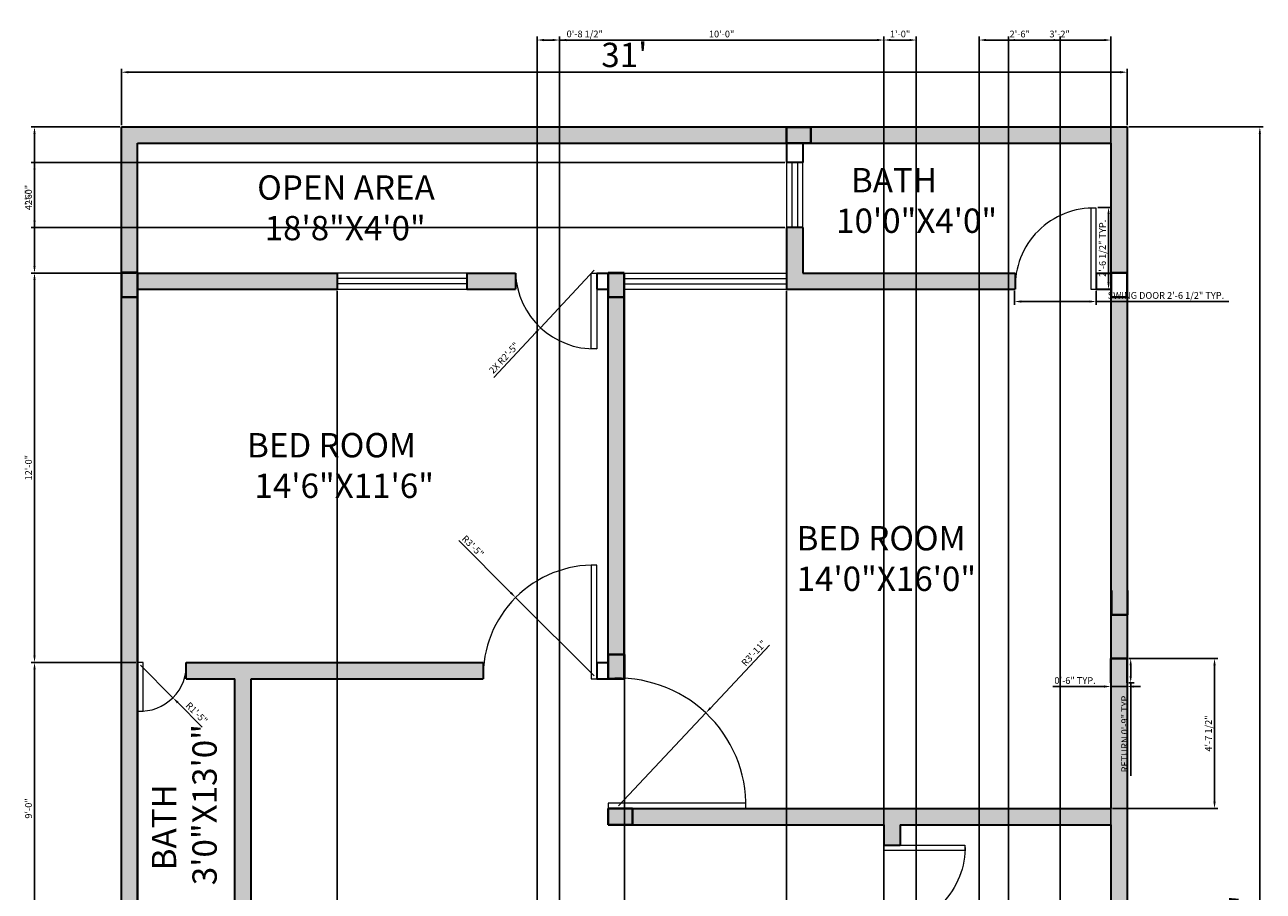
# Model space of a CAD drawing. Units: inches. Extents: x 5276 to 5736, y 3292 to 3966.
# Tile 3 of 3: x 5278 to 5736, y 3646 to 3966. Entities that reach past the tile are written whole.
import ezdxf

# ---------------------------------------------------------------- set-up
doc = ezdxf.new("R2010")
doc.units = ezdxf.units.IN
for name, color, linetype, lineweight in [('A-ANNO-DIMS', 2, 'Continuous', 18), ('A-AREA-IDEN', 7, 'Continuous', 18), ('A-COLS', 7, 'Continuous', 40), ('A-DOOR', 3, 'Continuous', 18), ('A-GLAZ', 4, 'Continuous', 18), ('A-WALL', 7, 'Continuous', 35)]:
    doc.layers.add(name, color=color, linetype=linetype, lineweight=lineweight)
doc.layers.add('A-COLS-PATT', color=244, linetype='Continuous', lineweight=13, true_color=0x991b1e)
doc.layers.add('A-WALL-PATT', color=141, linetype='Continuous', lineweight=13, true_color=0xadddf7)
doc.styles.get("Standard").update_dxf_attribs({"font": 'arial.ttf'})
doc.dimstyles.new('ISO-25', dxfattribs={"dimtxt": 2.5, "dimasz": 2.5, "dimexe": 1.25, "dimexo": 0.625, "dimtad": 1, "dimlunit": 3, "dimtxsty": 'Standard', "dimcen": 2.5, "dimadec": 0, "dimazin": 0, "dimtfac": 1, "dimtmove": 0, "dimatfit": 3, "dimfxl": 1, "dimarcsym": 0})

# ---------------------------------------------------------------- blocks, each defined once
blk = doc.blocks.new('*D16')
at = {"layer": 'A-ANNO-DIMS', "color": 0, "lineweight": -2, "transparency": 16777216}
for p, q in [((5314.13, 3928.87), (5314.13, 3949.75)), ((5686.13, 3928.87), (5686.13, 3949.75)), ((5316.63, 3948.5), (5683.63, 3948.5))]:
    blk.add_line(p, q, dxfattribs=at)
at = {"layer": 'A-ANNO-DIMS', "color": 0, "transparency": 16777216}
for points in [[(5316.63, 3948.92), (5316.63, 3948.09), (5314.13, 3948.5)], [(5683.63, 3948.92), (5683.63, 3948.09), (5686.13, 3948.5)]]:
    blk.add_solid(points, dxfattribs=at)
at = {"layer": 'Defpoints', "color": 0, "transparency": 16777216}
for p in [(5686.13, 3948.5), (5314.13, 3928.25), (5686.13, 3928.25)]:
    blk.add_point(p, dxfattribs=at)
at = {"layer": 'A-ANNO-DIMS', "color": 0, "transparency": 16777216, "insert": (5500.13, 3953.73), "char_height": 9, "attachment_point": 5}
blk.add_mtext("31'", dxfattribs=at)
blk = doc.blocks.new('*D17')
at = {"layer": 'A-ANNO-DIMS', "color": 0, "lineweight": -2, "transparency": 16777216}
for p, q in [((5686.75, 3928.25), (5736.45, 3928.25)), ((5735.2, 3925.75), (5735.2, 3328.75)), ((5686.75, 3326.25), (5736.45, 3326.25))]:
    blk.add_line(p, q, dxfattribs=at)
at = {"layer": 'A-ANNO-DIMS', "color": 0, "transparency": 16777216}
for points in [[(5734.78, 3925.75), (5735.62, 3925.75), (5735.2, 3928.25)], [(5734.78, 3328.75), (5735.62, 3328.75), (5735.2, 3326.25)]]:
    blk.add_solid(points, dxfattribs=at)
at = {"layer": 'Defpoints', "color": 0, "transparency": 16777216}
for p in [(5686.13, 3928.25), (5686.13, 3326.25), (5735.2, 3326.25)]:
    blk.add_point(p, dxfattribs=at)
at = {"layer": 'A-ANNO-DIMS', "color": 0, "transparency": 16777216, "insert": (5729.98, 3627.25), "char_height": 9, "attachment_point": 5, "rotation": 90}
blk.add_mtext('50\'-2"', dxfattribs=at)
blk = doc.blocks.new('PIER-6X9')
for p, q in [((0, 9), (6, 9)), ((0, 0), (0, 9)), ((6, 9), (6, 0)), ((6, 0), (0, 0))]:
    blk.add_line(p, q)
blk = doc.blocks.new('PIER-6X9-RETURN')
for p, q in [((0, 0), (0, 9)), ((6, 9), (6, 0)), ((6, 0), (0, 0))]:
    blk.add_line(p, q)
blk = doc.blocks.new('DOOR-SWING-30')
for p, q in [((0, 30), (-2, 30)), ((-2, 30), (-2, 0)), ((0, 0), (0, 30)), ((-2, 0), (0, 0))]:
    blk.add_line(p, q)
blk.add_arc((-1, 1), 29.02, 88.0251, 181.9749)
blk = doc.blocks.new('WINDOW-48X6')
for p, q in [((0, 6), (0, 0)), ((48, 6), (0, 6)), ((48, 0), (48, 6)), ((48, 4), (0, 4)), ((48, 2), (0, 2)), ((0, 0), (48, 0))]:
    blk.add_line(p, q)
blk = doc.blocks.new('*D24')
at = {"layer": 'A-ANNO-DIMS', "color": 0, "lineweight": -2, "transparency": 16777216}
for p, q in [((5686.71, 3731.69), (5688.68, 3731.69)), ((5687.43, 3729.19), (5687.43, 3725.19)), ((5686.71, 3722.69), (5688.68, 3722.69)), ((5687.43, 3722.69), (5687.43, 3688.31))]:
    blk.add_line(p, q, dxfattribs=at)
at = {"layer": 'A-ANNO-DIMS', "color": 0, "transparency": 16777216}
for points in [[(5687.02, 3729.19), (5687.85, 3729.19), (5687.43, 3731.69)], [(5687.02, 3725.19), (5687.85, 3725.19), (5687.43, 3722.69)]]:
    blk.add_solid(points, dxfattribs=at)
at = {"layer": 'Defpoints', "color": 0, "transparency": 16777216}
for p in [(5686.08, 3731.69), (5686.08, 3722.69), (5687.43, 3722.69)]:
    blk.add_point(p, dxfattribs=at)
at = {"layer": 'A-ANNO-DIMS', "color": 0, "transparency": 16777216, "insert": (5685.53, 3704.25), "char_height": 2.5, "attachment_point": 5, "rotation": 90}
blk.add_mtext('RETURN 0\'-9" TYP.', dxfattribs=at)
blk = doc.blocks.new('*D25')
at = {"layer": 'A-ANNO-DIMS', "color": 0, "lineweight": -2, "transparency": 16777216}
for p, q in [((5677.58, 3721.34), (5658.59, 3721.34)), ((5680.08, 3722.06), (5680.08, 3720.09)), ((5686.08, 3721.34), (5680.08, 3721.34)), ((5686.08, 3722.06), (5686.08, 3720.09)), ((5688.58, 3721.34), (5691.08, 3721.34))]:
    blk.add_line(p, q, dxfattribs=at)
at = {"layer": 'A-ANNO-DIMS', "color": 0, "transparency": 16777216}
for points in [[(5677.58, 3721.75), (5677.58, 3720.92), (5680.08, 3721.34)], [(5688.58, 3721.75), (5688.58, 3720.92), (5686.08, 3721.34)]]:
    blk.add_solid(points, dxfattribs=at)
at = {"layer": 'Defpoints', "color": 0, "transparency": 16777216}
for p in [(5680.08, 3722.69), (5680.08, 3721.34), (5686.08, 3722.69)]:
    blk.add_point(p, dxfattribs=at)
at = {"layer": 'A-ANNO-DIMS', "color": 0, "transparency": 16777216, "insert": (5666.84, 3723.24), "char_height": 2.5, "attachment_point": 5}
blk.add_mtext('0\'-6" TYP.', dxfattribs=at)
blk = doc.blocks.new('*D26')
at = {"layer": 'A-ANNO-DIMS', "color": 0, "lineweight": -2, "transparency": 16777216}
for p, q in [((5644.42, 3867.62), (5644.42, 3862.46)), ((5674.7, 3867.62), (5674.7, 3862.46)), ((5646.92, 3863.71), (5672.2, 3863.71)), ((5674.7, 3863.71), (5723.75, 3863.71))]:
    blk.add_line(p, q, dxfattribs=at)
at = {"layer": 'A-ANNO-DIMS', "color": 0, "transparency": 16777216}
for points in [[(5646.92, 3864.12), (5646.92, 3863.29), (5644.42, 3863.71)], [(5672.2, 3864.12), (5672.2, 3863.29), (5674.7, 3863.71)]]:
    blk.add_solid(points, dxfattribs=at)
at = {"layer": 'Defpoints', "color": 0, "transparency": 16777216}
for p in [(5644.42, 3868.25), (5674.7, 3868.25), (5674.7, 3863.71)]:
    blk.add_point(p, dxfattribs=at)
at = {"layer": 'A-ANNO-DIMS', "color": 0, "transparency": 16777216, "insert": (5700.47, 3865.63), "char_height": 2.5, "attachment_point": 5}
blk.add_mtext('SWING DOOR 2\'-6 1/2" TYP.', dxfattribs=at)
blk = doc.blocks.new('*D27')
at = {"layer": 'A-ANNO-DIMS', "color": 0, "lineweight": -2, "transparency": 16777216}
for p, q in [((5675.32, 3898.53), (5680.49, 3898.53)), ((5679.24, 3870.75), (5679.24, 3896.03)), ((5675.32, 3868.25), (5680.49, 3868.25))]:
    blk.add_line(p, q, dxfattribs=at)
at = {"layer": 'A-ANNO-DIMS', "color": 0, "transparency": 16777216}
for points in [[(5678.82, 3896.03), (5679.65, 3896.03), (5679.24, 3898.53)], [(5678.82, 3870.75), (5679.65, 3870.75), (5679.24, 3868.25)]]:
    blk.add_solid(points, dxfattribs=at)
at = {"layer": 'Defpoints', "color": 0, "transparency": 16777216}
for p in [(5674.7, 3898.53), (5679.24, 3898.53), (5674.7, 3868.25)]:
    blk.add_point(p, dxfattribs=at)
at = {"layer": 'A-ANNO-DIMS', "color": 0, "transparency": 16777216, "insert": (5677.32, 3883.39), "char_height": 2.5, "attachment_point": 5, "rotation": 90}
blk.add_mtext('2\'-6 1/2" TYP.', dxfattribs=at)
blk = doc.blocks.new('*D33')
at = {"layer": 'A-ANNO-DIMS', "color": 0, "lineweight": -2, "transparency": 16777216}
for p, q in [((5467.88, 3334.87), (5467.88, 3961.65)), ((5470.38, 3960.4), (5473.63, 3960.4)), ((5476.13, 3334.87), (5476.13, 3961.65)), ((5476.13, 3960.4), (5492.35, 3960.4))]:
    blk.add_line(p, q, dxfattribs=at)
at = {"layer": 'A-ANNO-DIMS', "color": 0, "transparency": 16777216}
for points in [[(5470.38, 3960.82), (5470.38, 3959.98), (5467.88, 3960.4)], [(5473.63, 3960.82), (5473.63, 3959.98), (5476.13, 3960.4)]]:
    blk.add_solid(points, dxfattribs=at)
at = {"layer": 'Defpoints', "color": 0, "transparency": 16777216}
for p in [(5476.13, 3960.4), (5467.88, 3334.25), (5476.13, 3334.25)]:
    blk.add_point(p, dxfattribs=at)
at = {"layer": 'A-ANNO-DIMS', "color": 0, "transparency": 16777216, "insert": (5485.49, 3962.32), "char_height": 2.5, "attachment_point": 5}
blk.add_mtext('0\'-8 1/2"', dxfattribs=at)
blk = doc.blocks.new('*D38')
at = {"layer": 'A-ANNO-DIMS', "color": 0, "lineweight": -2, "transparency": 16777216}
for p, q in [((5319.5, 3730.25), (5280.73, 3730.25)), ((5281.98, 3624.75), (5281.98, 3727.75)), ((5319.5, 3622.25), (5280.73, 3622.25))]:
    blk.add_line(p, q, dxfattribs=at)
at = {"layer": 'A-ANNO-DIMS', "color": 0, "transparency": 16777216}
for points in [[(5281.56, 3727.75), (5282.39, 3727.75), (5281.98, 3730.25)], [(5281.56, 3624.75), (5282.39, 3624.75), (5281.98, 3622.25)]]:
    blk.add_solid(points, dxfattribs=at)
at = {"layer": 'Defpoints', "color": 0, "transparency": 16777216}
for p in [(5281.98, 3730.25), (5320.13, 3730.25), (5320.13, 3622.25)]:
    blk.add_point(p, dxfattribs=at)
at = {"layer": 'A-ANNO-DIMS', "color": 0, "transparency": 16777216, "insert": (5280.08, 3676.25), "char_height": 2.5, "attachment_point": 5, "rotation": 90}
blk.add_mtext('9\'-0"', dxfattribs=at)
blk = doc.blocks.new('*D39')
at = {"layer": 'A-ANNO-DIMS', "color": 0, "lineweight": -2, "transparency": 16777216}
for p, q in [((5319.5, 3874.25), (5280.73, 3874.25)), ((5281.98, 3732.75), (5281.98, 3871.75)), ((5319.5, 3730.25), (5280.73, 3730.25))]:
    blk.add_line(p, q, dxfattribs=at)
at = {"layer": 'A-ANNO-DIMS', "color": 0, "transparency": 16777216}
for points in [[(5281.56, 3871.75), (5282.39, 3871.75), (5281.98, 3874.25)], [(5281.56, 3732.75), (5282.39, 3732.75), (5281.98, 3730.25)]]:
    blk.add_solid(points, dxfattribs=at)
at = {"layer": 'Defpoints', "color": 0, "transparency": 16777216}
for p in [(5281.98, 3874.25), (5320.13, 3874.25), (5320.13, 3730.25)]:
    blk.add_point(p, dxfattribs=at)
at = {"layer": 'A-ANNO-DIMS', "color": 0, "transparency": 16777216, "insert": (5280.08, 3802.25), "char_height": 2.5, "attachment_point": 5, "rotation": 90}
blk.add_mtext('12\'-0"', dxfattribs=at)
blk = doc.blocks.new('*D40')
at = {"layer": 'A-ANNO-DIMS', "color": 0, "lineweight": -2, "transparency": 16777216}
for p, q in [((5313.5, 3928.25), (5280.73, 3928.25)), ((5281.98, 3876.75), (5281.98, 3925.75)), ((5319.5, 3874.25), (5280.73, 3874.25))]:
    blk.add_line(p, q, dxfattribs=at)
at = {"layer": 'A-ANNO-DIMS', "color": 0, "transparency": 16777216}
for points in [[(5281.56, 3925.75), (5282.39, 3925.75), (5281.98, 3928.25)], [(5281.56, 3876.75), (5282.39, 3876.75), (5281.98, 3874.25)]]:
    blk.add_solid(points, dxfattribs=at)
at = {"layer": 'Defpoints', "color": 0, "transparency": 16777216}
for p in [(5281.98, 3928.25), (5314.13, 3928.25), (5320.13, 3874.25)]:
    blk.add_point(p, dxfattribs=at)
at = {"layer": 'A-ANNO-DIMS', "color": 0, "transparency": 16777216, "insert": (5280.08, 3901.25), "char_height": 2.5, "attachment_point": 5, "rotation": 90}
blk.add_mtext('4\'-6"', dxfattribs=at)
blk = doc.blocks.new('*D41')
at = {"layer": 'A-ANNO-DIMS', "color": 0, "lineweight": -2, "transparency": 16777216}
for p, q in [((5476.13, 3382.87), (5476.13, 3961.65)), ((5478.63, 3960.4), (5593.62, 3960.4)), ((5596.12, 3382.87), (5596.12, 3961.65))]:
    blk.add_line(p, q, dxfattribs=at)
at = {"layer": 'A-ANNO-DIMS', "color": 0, "transparency": 16777216}
for points in [[(5478.63, 3960.82), (5478.63, 3959.98), (5476.13, 3960.4)], [(5593.62, 3960.82), (5593.62, 3959.98), (5596.12, 3960.4)]]:
    blk.add_solid(points, dxfattribs=at)
at = {"layer": 'Defpoints', "color": 0, "transparency": 16777216}
for p in [(5596.12, 3960.4), (5476.13, 3382.25), (5596.12, 3382.25)]:
    blk.add_point(p, dxfattribs=at)
at = {"layer": 'A-ANNO-DIMS', "color": 0, "transparency": 16777216, "insert": (5536.12, 3962.3), "char_height": 2.5, "attachment_point": 5}
blk.add_mtext('10\'-0"', dxfattribs=at)
blk = doc.blocks.new('*D44')
at = {"layer": 'A-ANNO-DIMS', "color": 0, "lineweight": -2, "transparency": 16777216}
for p, q in [((5642.17, 3450.24), (5642.17, 3961.65)), ((5644.67, 3960.4), (5677.63, 3960.4)), ((5680.13, 3450.24), (5680.13, 3961.65))]:
    blk.add_line(p, q, dxfattribs=at)
at = {"layer": 'A-ANNO-DIMS', "color": 0, "transparency": 16777216}
for points in [[(5644.67, 3960.82), (5644.67, 3959.98), (5642.17, 3960.4)], [(5677.63, 3960.82), (5677.63, 3959.98), (5680.13, 3960.4)]]:
    blk.add_solid(points, dxfattribs=at)
at = {"layer": 'Defpoints', "color": 0, "transparency": 16777216}
for p in [(5680.13, 3960.4), (5642.17, 3449.62), (5680.13, 3449.62)]:
    blk.add_point(p, dxfattribs=at)
at = {"layer": 'A-ANNO-DIMS', "color": 0, "transparency": 16777216, "insert": (5661.15, 3962.3), "char_height": 2.5, "attachment_point": 5}
blk.add_mtext('3\'-2"', dxfattribs=at)
blk = doc.blocks.new('*D47')
at = {"layer": 'A-ANNO-DIMS', "color": 0, "lineweight": -2, "transparency": 16777216}
for p, q in [((5596.12, 3450.24), (5596.12, 3961.65)), ((5598.62, 3960.4), (5605.62, 3960.4)), ((5608.12, 3450.24), (5608.12, 3961.65))]:
    blk.add_line(p, q, dxfattribs=at)
at = {"layer": 'A-ANNO-DIMS', "color": 0, "transparency": 16777216}
for points in [[(5598.62, 3960.82), (5598.62, 3959.98), (5596.12, 3960.4)], [(5605.62, 3960.82), (5605.62, 3959.98), (5608.12, 3960.4)]]:
    blk.add_solid(points, dxfattribs=at)
at = {"layer": 'Defpoints', "color": 0, "transparency": 16777216}
for p in [(5608.12, 3960.4), (5596.12, 3449.62), (5608.12, 3449.62)]:
    blk.add_point(p, dxfattribs=at)
at = {"layer": 'A-ANNO-DIMS', "color": 0, "transparency": 16777216, "insert": (5602.12, 3962.3), "char_height": 2.5, "attachment_point": 5}
blk.add_mtext('1\'-0"', dxfattribs=at)
blk = doc.blocks.new('*D52')
at = {"layer": 'A-ANNO-DIMS', "color": 0, "lineweight": -2, "transparency": 16777216}
for p, q in [((5631.38, 3568.87), (5631.38, 3961.65)), ((5633.88, 3960.4), (5658.88, 3960.4)), ((5661.38, 3568.87), (5661.38, 3961.65))]:
    blk.add_line(p, q, dxfattribs=at)
at = {"layer": 'A-ANNO-DIMS', "color": 0, "transparency": 16777216}
for points in [[(5633.88, 3960.82), (5633.88, 3959.98), (5631.38, 3960.4)], [(5658.88, 3960.82), (5658.88, 3959.98), (5661.38, 3960.4)]]:
    blk.add_solid(points, dxfattribs=at)
at = {"layer": 'Defpoints', "color": 0, "transparency": 16777216}
for p in [(5661.38, 3960.4), (5631.38, 3568.25), (5661.38, 3568.25)]:
    blk.add_point(p, dxfattribs=at)
at = {"layer": 'A-ANNO-DIMS', "color": 0, "transparency": 16777216, "insert": (5646.38, 3962.3), "char_height": 2.5, "attachment_point": 5}
blk.add_mtext('2\'-6"', dxfattribs=at)
blk = doc.blocks.new('*D53')
at = {"layer": 'A-ANNO-DIMS', "color": 0, "lineweight": -2, "transparency": 16777216}
for p, q in [((5320.13, 3867.62), (5320.13, 3292.85)), ((5393.93, 3867.62), (5393.93, 3292.85)), ((5322.63, 3294.1), (5391.43, 3294.1))]:
    blk.add_line(p, q, dxfattribs=at)
at = {"layer": 'A-ANNO-DIMS', "color": 0, "transparency": 16777216}
for points in [[(5322.63, 3294.52), (5322.63, 3293.68), (5320.13, 3294.1)], [(5391.43, 3294.52), (5391.43, 3293.68), (5393.93, 3294.1)]]:
    blk.add_solid(points, dxfattribs=at)
at = {"layer": 'Defpoints', "color": 0, "transparency": 16777216}
for p in [(5320.13, 3868.25), (5393.93, 3868.25), (5393.93, 3294.1)]:
    blk.add_point(p, dxfattribs=at)
at = {"layer": 'A-ANNO-DIMS', "color": 0, "transparency": 16777216, "insert": (5357.03, 3296), "char_height": 2.5, "attachment_point": 5}
blk.add_mtext('6\'-2"', dxfattribs=at)
blk = doc.blocks.new('*D54')
at = {"layer": 'A-ANNO-DIMS', "color": 0, "lineweight": -2, "transparency": 16777216}
for p, q in [((5500.14, 3867.62), (5500.14, 3292.85)), ((5560.13, 3867.62), (5560.13, 3292.85)), ((5502.64, 3294.1), (5557.63, 3294.1))]:
    blk.add_line(p, q, dxfattribs=at)
at = {"layer": 'A-ANNO-DIMS', "color": 0, "transparency": 16777216}
for points in [[(5502.64, 3294.52), (5502.64, 3293.68), (5500.14, 3294.1)], [(5557.63, 3294.52), (5557.63, 3293.68), (5560.13, 3294.1)]]:
    blk.add_solid(points, dxfattribs=at)
at = {"layer": 'Defpoints', "color": 0, "transparency": 16777216}
for p in [(5500.14, 3868.25), (5560.13, 3868.25), (5560.13, 3294.1)]:
    blk.add_point(p, dxfattribs=at)
at = {"layer": 'A-ANNO-DIMS', "color": 0, "transparency": 16777216, "insert": (5530.13, 3296), "char_height": 2.5, "attachment_point": 5}
blk.add_mtext('5\'-0"', dxfattribs=at)
blk = doc.blocks.new('*D55')
at = {"layer": 'A-ANNO-DIMS', "color": 0, "lineweight": -2, "transparency": 16777216}
for p, q in [((5559.5, 3915.07), (5280.73, 3915.07)), ((5281.98, 3893.57), (5281.98, 3912.57)), ((5559.5, 3891.07), (5280.73, 3891.07))]:
    blk.add_line(p, q, dxfattribs=at)
at = {"layer": 'A-ANNO-DIMS', "color": 0, "transparency": 16777216}
for points in [[(5281.56, 3912.57), (5282.39, 3912.57), (5281.98, 3915.07)], [(5281.56, 3893.57), (5282.39, 3893.57), (5281.98, 3891.07)]]:
    blk.add_solid(points, dxfattribs=at)
at = {"layer": 'Defpoints', "color": 0, "transparency": 16777216}
for p in [(5281.98, 3915.07), (5560.13, 3915.07), (5560.13, 3891.07)]:
    blk.add_point(p, dxfattribs=at)
at = {"layer": 'A-ANNO-DIMS', "color": 0, "transparency": 16777216, "insert": (5280.08, 3903.07), "char_height": 2.5, "attachment_point": 5, "rotation": 90}
blk.add_mtext('2\'-0"', dxfattribs=at)
blk = doc.blocks.new('*D56')
at = {"layer": 'A-ANNO-DIMS', "color": 0, "lineweight": -2, "transparency": 16777216}
for p, q in [((5686.71, 3731.69), (5719.69, 3731.69)), ((5718.44, 3678.75), (5718.44, 3729.19)), ((5680.75, 3676.25), (5719.69, 3676.25))]:
    blk.add_line(p, q, dxfattribs=at)
at = {"layer": 'A-ANNO-DIMS', "color": 0, "transparency": 16777216}
for points in [[(5718.02, 3729.19), (5718.86, 3729.19), (5718.44, 3731.69)], [(5718.02, 3678.75), (5718.86, 3678.75), (5718.44, 3676.25)]]:
    blk.add_solid(points, dxfattribs=at)
at = {"layer": 'Defpoints', "color": 0, "transparency": 16777216}
for p in [(5686.08, 3731.69), (5718.44, 3731.69), (5680.13, 3676.25)]:
    blk.add_point(p, dxfattribs=at)
at = {"layer": 'A-ANNO-DIMS', "color": 0, "transparency": 16777216, "insert": (5716.52, 3703.97), "char_height": 2.5, "attachment_point": 5, "rotation": 90}
blk.add_mtext('4\'-7 1/2"', dxfattribs=at)
blk = doc.blocks.new('*D58')
at = {"layer": 'A-ANNO-DIMS', "color": 0, "lineweight": -2, "transparency": 16777216}
for p, q in [((5553.88, 3736.64), (5532, 3713.4)), ((5497.96, 3677.24), (5530.29, 3711.58))]:
    blk.add_line(p, q, dxfattribs=at)
at = {"layer": 'A-ANNO-DIMS', "color": 0, "transparency": 16777216}
blk.add_solid([(5531.7, 3713.69), (5532.3, 3713.12), (5530.29, 3711.58)], dxfattribs=at)
at = {"layer": 'Defpoints', "color": 0, "transparency": 16777216}
for p in [(5530.29, 3711.58), (5497.96, 3677.24)]:
    blk.add_point(p, dxfattribs=at)
at = {"layer": 'A-ANNO-DIMS', "color": 0, "transparency": 16777216, "insert": (5548.3, 3733.49), "char_height": 2.5, "attachment_point": 5, "rotation": 46.7277}
blk.add_mtext('R3\'-11"', dxfattribs=at)
blk = doc.blocks.new('*D60')
at = {"layer": 'A-ANNO-DIMS', "color": 0, "lineweight": -2, "transparency": 16777216}
for p, q in [((5438.89, 3775.29), (5458.16, 3756.02)), ((5488.93, 3725.25), (5459.93, 3754.25))]:
    blk.add_line(p, q, dxfattribs=at)
at = {"layer": 'A-ANNO-DIMS', "color": 0, "transparency": 16777216}
blk.add_solid([(5458.46, 3756.31), (5457.87, 3755.72), (5459.93, 3754.25)], dxfattribs=at)
at = {"layer": 'Defpoints', "color": 0, "transparency": 16777216}
for p in [(5459.93, 3754.25), (5488.93, 3725.25)]:
    blk.add_point(p, dxfattribs=at)
at = {"layer": 'A-ANNO-DIMS', "color": 0, "transparency": 16777216, "insert": (5443.87, 3772.99), "char_height": 2.5, "attachment_point": 5, "rotation": 315.0004}
blk.add_mtext('R3\'-5"', dxfattribs=at)
blk = doc.blocks.new('*D62')
at = {"layer": 'A-ANNO-DIMS', "color": 0, "lineweight": -2, "transparency": 16777216}
for p, q in [((5488.93, 3875.25), (5469.13, 3854.04)), ((5451.89, 3835.57), (5467.42, 3852.21))]:
    blk.add_line(p, q, dxfattribs=at)
at = {"layer": 'A-ANNO-DIMS', "color": 0, "transparency": 16777216}
blk.add_solid([(5467.12, 3852.49), (5467.73, 3851.92), (5469.13, 3854.04)], dxfattribs=at)
at = {"layer": 'Defpoints', "color": 0, "transparency": 16777216}
for p in [(5488.93, 3875.25), (5469.13, 3854.04)]:
    blk.add_point(p, dxfattribs=at)
at = {"layer": 'A-ANNO-DIMS', "color": 0, "transparency": 16777216, "insert": (5455.86, 3842.61), "char_height": 2.5, "attachment_point": 5, "rotation": 46.9744}
blk.add_mtext('2X R2\'-5"', dxfattribs=at)
blk = doc.blocks.new('*D66')
at = {"layer": 'A-ANNO-DIMS', "color": 0, "lineweight": -2, "transparency": 16777216}
for p, q in [((5321.13, 3729.25), (5333.17, 3717.21)), ((5344.03, 3706.35), (5334.94, 3715.44))]:
    blk.add_line(p, q, dxfattribs=at)
at = {"layer": 'A-ANNO-DIMS', "color": 0, "transparency": 16777216}
blk.add_solid([(5335.23, 3715.73), (5334.64, 3715.15), (5333.17, 3717.21)], dxfattribs=at)
at = {"layer": 'Defpoints', "color": 0, "transparency": 16777216}
for p in [(5321.13, 3729.25), (5333.17, 3717.21)]:
    blk.add_point(p, dxfattribs=at)
at = {"layer": 'A-ANNO-DIMS', "color": 0, "transparency": 16777216, "insert": (5341.74, 3711.33), "char_height": 2.5, "attachment_point": 5, "rotation": 315.0009}
blk.add_mtext('R1\'-5"', dxfattribs=at)

msp = doc.modelspace()

# ---------------------------------------------------------------- hatches: boundary and pattern name
at = {"layer": 'A-COLS-PATT'}
h = msp.add_hatch(color=256, dxfattribs=at)
h.dxf.hatch_style = 1
h.paths.add_polyline_path([(5320.127, 3874.381), (5314.129, 3874.381), (5314.129, 3865.381), (5320.127, 3865.381)])
h.paths.add_polyline_path([(5500.127, 3874.249), (5494.136, 3874.249), (5494.136, 3865.268), (5500.127, 3865.268)])
h.paths.add_polyline_path([(5500.127, 3733.242), (5494.138, 3733.242), (5494.138, 3724.249), (5500.127, 3724.249)])
h.paths.add_polyline_path([(5569.096, 3928.221), (5560.096, 3928.221), (5560.096, 3922.249), (5560.127, 3922.249), (5566.127, 3922.23), (5566.127, 3922.249), (5569.096, 3922.249)])
h.paths.add_polyline_path([(5686.127, 3747.872), (5680.127, 3747.872), (5680.127, 3731.687), (5686.127, 3731.687)])
h.paths.add_polyline_path([(5503.112, 3676.236), (5494.127, 3676.236), (5494.127, 3670.249), (5503.112, 3670.249)])
h.paths.add_polyline_path([(5320.127, 3514.161), (5314.167, 3514.161), (5314.167, 3505.161), (5320.127, 3505.161)])
h.paths.add_polyline_path([(5320.127, 3391.305), (5314.138, 3391.305), (5314.138, 3382.305), (5320.127, 3382.305)])
h.paths.add_polyline_path([(5476.116, 3391.239), (5470.127, 3391.239), (5470.127, 3382.249), (5476.116, 3382.249)])
h.paths.add_polyline_path([(5476.1, 3508.238), (5470.127, 3508.238), (5470.127, 3499.238), (5476.1, 3499.238)])
h.paths.add_polyline_path([(5359.148, 3568.249), (5350.148, 3568.249), (5350.148, 3562.297), (5359.148, 3562.297)])
h.paths.add_polyline_path([(5476.127, 3568.222), (5467.137, 3568.222), (5467.137, 3562.249), (5476.127, 3562.249)])
h.paths.add_polyline_path([(5602.119, 3571.238), (5596.127, 3571.238), (5596.127, 3562.249), (5602.119, 3562.249)])
h.paths.add_polyline_path([(5686.112, 3571.26), (5680.127, 3571.26), (5680.127, 3568.249), (5680.112, 3562.26), (5686.112, 3562.26)])
h.paths.add_polyline_path([(5686.094, 3508.787), (5680.127, 3508.787), (5680.127, 3499.787), (5686.094, 3499.787)])
h = msp.add_hatch(color=256, dxfattribs=at)
h.dxf.hatch_style = 1
h.paths.add_polyline_path([(5686.083, 3731.687), (5680.127, 3731.687), (5680.127, 3722.687), (5686.083, 3722.687)])
h.paths.add_polyline_path([(5686.127, 3756.872), (5680.29, 3756.872), (5680.29, 3747.872), (5686.127, 3747.872)])
at = {"layer": 'A-WALL-PATT'}
h = msp.add_hatch(color=256, dxfattribs=at)
h.dxf.hatch_style = 1
h.paths.add_polyline_path([(5560.096, 3928.249), (5314.127, 3928.249), (5314.127, 3874.381), (5320.127, 3874.381), (5320.127, 3922.249), (5560.096, 3922.249)])
h.paths.add_polyline_path([(5500.127, 3865.268), (5494.127, 3865.268), (5494.127, 3733.242), (5500.127, 3733.242)])
h.paths.add_polyline_path([(5644.696, 3874.249), (5566.127, 3874.249), (5566.127, 3891.071), (5560.127, 3891.071), (5560.127, 3868.249), (5644.696, 3868.249)])
h.paths.add_polyline_path([(5686.127, 3928.249), (5569.096, 3928.249), (5569.096, 3922.249), (5680.127, 3922.249), (5680.127, 3874.262), (5686.127, 3874.262)])
h.paths.add_polyline_path([(5686.127, 3865.262), (5680.127, 3865.262), (5680.127, 3756.872), (5686.127, 3756.872)])
h.paths.add_polyline_path([(5393.929, 3874.249), (5320.129, 3874.249), (5320.129, 3868.249), (5393.929, 3868.249)])
h.paths.add_polyline_path([(5459.929, 3874.249), (5441.929, 3874.249), (5441.929, 3868.249), (5459.929, 3868.249)])
h.paths.add_polyline_path([(5447.929, 3730.249), (5338.127, 3730.249), (5338.127, 3724.249), (5356.127, 3724.249), (5356.127, 3628.249), (5344.74, 3628.249), (5344.74, 3622.249), (5356.127, 3622.249), (5356.127, 3598.249), (5362.127, 3598.249), (5362.127, 3724.249), (5447.929, 3724.249)])
h.paths.add_polyline_path([(5320.127, 3865.381), (5314.127, 3865.381), (5314.127, 3514.249), (5320.127, 3514.249), (5320.127, 3568.249)])
h.paths.add_polyline_path([(5686.127, 3722.687), (5680.127, 3722.687), (5680.127, 3676.249), (5503.112, 3676.249), (5503.112, 3670.249), (5596.127, 3670.249), (5596.127, 3662.687), (5602.127, 3662.687), (5602.127, 3670.249), (5680.127, 3670.249), (5680.127, 3571.26), (5686.127, 3571.26)])
h.paths.add_polyline_path([(5596.119, 3568.249), (5536.127, 3568.249), (5536.127, 3562.249), (5543.142, 3562.249), (5596.119, 3562.249)])
h.paths.add_polyline_path([(5602.127, 3632.687), (5596.127, 3632.687), (5596.127, 3571.238), (5602.127, 3571.238)])
h.paths.add_polyline_path([(5631.383, 3568.249), (5602.127, 3568.249), (5602.127, 3562.249), (5631.383, 3562.249)])
h.paths.add_polyline_path([(5680.112, 3568.249), (5661.383, 3568.249), (5661.383, 3562.249), (5680.112, 3562.249)])
h.paths.add_polyline_path([(5686.127, 3562.26), (5680.127, 3562.26), (5680.127, 3508.787), (5686.127, 3508.787)])
h.paths.add_polyline_path([(5686.127, 3499.787), (5680.127, 3499.787), (5680.127, 3391.131), (5686.127, 3391.131)])
h.paths.add_polyline_path([(5686.127, 3382.131), (5680.127, 3382.131), (5680.127, 3328.249), (5686.127, 3328.249)])
h.paths.add_polyline_path([(5320.127, 3505.161), (5314.127, 3505.161), (5314.127, 3391.305), (5320.127, 3391.305)])
h.paths.add_polyline_path([(5344.127, 3388.249), (5320.138, 3388.249), (5320.138, 3382.249), (5344.127, 3382.249)])
h.paths.add_polyline_path([(5428.127, 3388.249), (5392.127, 3388.249), (5392.127, 3382.249), (5428.127, 3382.249)])
h.paths.add_polyline_path([(5476.127, 3499.238), (5470.127, 3499.238), (5470.127, 3397.332), (5470.127, 3391.239), (5476.127, 3391.239), (5476.127, 3397.332)])
h.paths.add_polyline_path([(5446.127, 3517.875), (5440.127, 3517.875), (5440.127, 3514.249), (5356.127, 3514.249), (5356.127, 3528.065), (5350.127, 3528.065), (5350.127, 3508.249), (5446.127, 3508.249)])
h.paths.add_polyline_path([(5356.127, 3562.249), (5350.127, 3562.249), (5350.127, 3552.065), (5356.127, 3552.065)])
h.paths.add_polyline_path([(5467.137, 3568.249), (5359.148, 3568.249), (5359.148, 3562.249), (5440.127, 3562.249), (5440.127, 3547.875), (5446.127, 3547.875), (5446.127, 3562.249), (5467.137, 3562.249)])

# ---------------------------------------------------------------- linework, layer by layer
at = {"layer": 'A-DOOR'}
for p, q in [((5487.929, 3846.249), (5487.929, 3874.249)), ((5487.929, 3874.249), (5489.929, 3874.249)), ((5489.929, 3874.249), (5489.929, 3846.249)), ((5489.929, 3846.249), (5487.929, 3846.249)), ((5489.929, 3766.249), (5487.929, 3766.249)), ((5487.929, 3766.249), (5487.929, 3724.249)), ((5489.929, 3724.249), (5489.929, 3766.249)), ((5320.127, 3730.249), (5320.127, 3712.249)), ((5322.127, 3730.249), (5320.127, 3730.249)), ((5322.127, 3712.249), (5322.127, 3730.249)), ((5487.929, 3724.249), (5489.929, 3724.249)), ((5320.127, 3712.249), (5322.127, 3712.249)), ((5545.112, 3678.236), (5494.127, 3678.236)), ((5494.127, 3678.236), (5494.127, 3676.249)), ((5503.112, 3676.236), (5545.112, 3676.236)), ((5545.112, 3676.236), (5545.112, 3678.236))]:
    msp.add_line(p, q, dxfattribs=at)
for centre, radius, start, end in [((5488.929, 3875.249), 29.017, 181.97493, 271.97493), ((5488.929, 3725.249), 41.012, 88.60282, 181.39718), ((5321.127, 3729.249), 17.029, 266.63354, 3.36646), ((5497.96, 3677.243), 47.162, 358.79289, 94.66181)]:
    msp.add_arc(centre, radius, start, end, dxfattribs=at)
at = {"layer": 'A-GLAZ'}
for p, q in [((5560.127, 3915.071), (5560.127, 3891.071)), ((5566.127, 3915.071), (5560.127, 3915.071)), ((5562.127, 3915.071), (5562.127, 3891.071)), ((5564.127, 3915.071), (5564.127, 3891.071)), ((5566.127, 3891.071), (5566.127, 3915.071)), ((5560.127, 3891.071), (5566.127, 3891.071)), ((5500.136, 3868.249), (5500.127, 3874.249)), ((5500.127, 3874.249), (5560.127, 3874.249)), ((5500.127, 3874.249), (5560.127, 3874.249)), ((5500.127, 3872.249), (5560.127, 3872.249)), ((5560.127, 3874.249), (5560.127, 3868.249)), ((5500.127, 3870.249), (5560.127, 3870.249)), ((5500.136, 3868.249), (5560.127, 3868.249))]:
    msp.add_line(p, q, dxfattribs=at)
at = {"layer": 'A-WALL'}
for p, q in [((5314.127, 3928.249), (5686.127, 3928.249)), ((5314.127, 3328.249), (5314.127, 3928.249)), ((5686.127, 3928.249), (5686.127, 3328.249)), ((5320.127, 3922.249), (5560.127, 3922.249)), ((5320.127, 3568.249), (5320.127, 3922.249)), ((5560.127, 3922.249), (5560.127, 3915.071)), ((5566.127, 3922.249), (5566.127, 3915.071)), ((5566.127, 3922.249), (5680.127, 3922.249)), ((5680.127, 3922.249), (5680.127, 3874.249)), ((5566.127, 3915.071), (5560.127, 3915.071)), ((5566.127, 3891.071), (5560.127, 3891.071)), ((5560.127, 3891.071), (5560.127, 3868.249)), ((5566.127, 3891.071), (5566.127, 3874.249)), ((5320.127, 3874.249), (5393.929, 3874.249)), ((5393.929, 3874.249), (5393.929, 3868.249)), ((5441.929, 3874.249), (5441.929, 3868.249)), ((5441.929, 3874.249), (5459.929, 3874.249)), ((5459.929, 3874.249), (5459.929, 3868.249)), ((5489.929, 3874.249), (5489.929, 3868.249)), ((5489.929, 3874.249), (5500.127, 3874.249)), ((5494.127, 3724.249), (5494.127, 3874.249)), ((5500.127, 3724.249), (5500.127, 3874.249)), ((5566.127, 3874.249), (5644.696, 3874.249)), ((5644.696, 3874.249), (5644.696, 3868.249)), ((5674.696, 3874.249), (5674.696, 3868.249)), ((5674.696, 3874.249), (5680.127, 3874.249)), ((5680.127, 3874.249), (5680.127, 3676.249)), ((5320.127, 3868.249), (5393.929, 3868.249)), ((5441.929, 3868.249), (5459.929, 3868.249)), ((5489.929, 3868.249), (5494.127, 3868.249)), ((5560.127, 3868.249), (5644.696, 3868.249)), ((5674.696, 3868.249), (5680.127, 3868.249)), ((5338.127, 3730.249), (5447.929, 3730.249)), ((5338.127, 3724.249), (5338.127, 3730.249)), ((5447.929, 3730.249), (5447.929, 3724.249)), ((5489.929, 3730.249), (5489.929, 3724.249)), ((5489.929, 3730.249), (5494.127, 3730.249)), ((5338.127, 3724.249), (5356.127, 3724.249)), ((5356.127, 3628.249), (5356.127, 3724.249)), ((5362.127, 3724.249), (5447.929, 3724.249)), ((5362.127, 3598.249), (5362.127, 3724.249)), ((5489.929, 3724.249), (5500.127, 3724.249)), ((5494.127, 3676.249), (5680.127, 3676.249)), ((5494.127, 3670.249), (5494.127, 3676.249)), ((5494.127, 3670.249), (5596.127, 3670.249)), ((5596.127, 3670.249), (5596.127, 3662.687)), ((5602.127, 3670.249), (5602.127, 3662.687)), ((5602.127, 3670.249), (5680.127, 3670.249)), ((5680.127, 3670.249), (5680.127, 3568.249)), ((5596.127, 3662.687), (5602.127, 3662.687))]:
    msp.add_line(p, q, dxfattribs=at)

# ---------------------------------------------------------------- block references
at = {"layer": 'A-COLS'}
for name, p, rotation in [('PIER-6X9', (5560.096, 3928.221), 270.0000000000053), ('PIER-6X9', (5500.136, 3874.268), 180), ('PIER-6X9', (5686.159, 3874.262), 180), ('PIER-6X9', (5500.138, 3733.242), 180), ('PIER-6X9-RETURN', (5686.083, 3731.687), 180), ('PIER-6X9', (5494.112, 3676.236), 269.9999999999893)]:
    msp.add_blockref(name, p, dxfattribs=dict(at, rotation=rotation))
for name, p in [('PIER-6X9', (5314.129, 3865.381)), ('PIER-6X9-RETURN', (5680.29, 3747.872))]:
    msp.add_blockref(name, p, dxfattribs=at)
at = {"layer": 'A-DOOR'}
msp.add_blockref('DOOR-SWING-30', (5674.696, 3868.249), dxfattribs=at)
at = {"layer": 'A-DOOR', "extrusion": (0, 0, -1), "zscale": -1, "rotation": 89.99999999999642}
msp.add_blockref('DOOR-SWING-30', (-5596.127, 3662.687), dxfattribs=at)
at = {"layer": 'A-GLAZ'}
msp.add_blockref('WINDOW-48X6', (5393.929, 3868.249), dxfattribs=at)

# ---------------------------------------------------------------- texts
at = {"layer": 'A-AREA-IDEN', "char_height": 9, "attachment_point": 1}
for s, insert in [('  BATH\\P10\'0"X4\'0"', (5578.456, 3913.096)), (' OPEN AREA\\P  18\'8"X4\'0"', (5361.591, 3910.362)), ('  BED ROOM\\P   14\'6"X11\'6"', (5355.079, 3815.08)), ('  BED ROOM\\P  14\'0"X16\'0"', (5558.362, 3780.686))]:
    msp.add_mtext_dynamic_manual_height_columns(s, width=110.27411, gutter_width=12.5, heights=[0], dxfattribs=dict(at, insert=insert))
at = {"layer": 'A-AREA-IDEN', "insert": (5325.372, 3645.126), "char_height": 9, "attachment_point": 1, "rotation": 90}
msp.add_mtext_dynamic_manual_height_columns('   BATH\\P 3\'0"X13\'0"', width=110.27411, gutter_width=12.5, heights=[0], dxfattribs=at)

# ---------------------------------------------------------------- dimensions: what is measured, and where the dimension line sits
at = {"layer": 'A-ANNO-DIMS'}
for base, p1, p2, override, picture, middle in [((5476.126509, 3960.399113), (5467.876509, 3334.249113), (5476.126509, 3334.249113), {"dimdec": 1, "dimlfac": 1, "dimrnd": 0, "dimzin": 1, "dimdsep": 46, "dimlunit": 4, "dimfrac": 2}, '*D33', (5485.487013775, 3962.316746015)), ((5596.119, 3960.399), (5476.127, 3382.249), (5596.119, 3382.249), {"dimdec": 1, "dimlfac": 1, "dimrnd": 0, "dimzin": 1, "dimdsep": 46, "dimlunit": 4, "dimfrac": 2}, '*D41', (5536.123, 3962.301)), ((5608.119, 3960.399), (5596.119, 3449.615), (5608.119, 3449.615), {"dimdec": 1, "dimlfac": 1, "dimrnd": 0, "dimzin": 1, "dimdsep": 46, "dimlunit": 4, "dimfrac": 2}, '*D47', (5602.119, 3962.301)), ((5661.383, 3960.399), (5631.383, 3568.249), (5661.383, 3568.249), {"dimdec": 1, "dimlfac": 1, "dimrnd": 0, "dimzin": 1, "dimdsep": 46, "dimlunit": 4, "dimfrac": 2}, '*D52', (5646.383, 3962.301)), ((5680.127, 3960.399), (5642.172, 3449.615), (5680.127, 3449.615), {"dimdec": 1, "dimlfac": 1, "dimrnd": 0, "dimzin": 1, "dimdsep": 46, "dimlunit": 4, "dimfrac": 2}, '*D44', (5661.149, 3962.301)), ((5686.127, 3948.502), (5314.127, 3928.249), (5686.127, 3928.249), {"dimtxt": 9, "dimclrd": 0, "dimclre": 0, "dimclrt": 0}, '*D16', (5500.127, 3953.725)), ((5393.929, 3294.099), (5320.127, 3868.249), (5393.929, 3868.249), {"dimdec": 1, "dimlfac": 1, "dimrnd": 0, "dimzin": 1, "dimdsep": 46, "dimlunit": 4, "dimfrac": 2}, '*D53', (5357.028, 3296.001)), ((5560.127, 3294.099), (5500.136, 3868.249), (5560.127, 3868.249), {"dimdec": 1, "dimlfac": 1, "dimrnd": 0, "dimzin": 1, "dimdsep": 46, "dimlunit": 4, "dimfrac": 2}, '*D54', (5530.131, 3296.001))]:
    dim = msp.add_linear_dim(base=base, p1=p1, p2=p2, dimstyle='ISO-25', override=override, dxfattribs=at)
    dim.commit()
    dim.dimension.update_dxf_attribs({"geometry": picture, "text_midpoint": middle})
for base, p1, p2, override, picture, middle in [((5281.977, 3928.249), (5320.127, 3874.249), (5314.127, 3928.249), {"dimdec": 1, "dimlfac": 1, "dimrnd": 0, "dimzin": 1, "dimdsep": 46, "dimlunit": 4, "dimfrac": 2}, '*D40', (5280.075, 3901.249)), ((5735.2, 3326.249), (5686.127, 3928.249), (5686.127, 3326.249), {"dimtxt": 9, "dimclrd": 0, "dimclre": 0, "dimclrt": 0}, '*D17', (5729.98, 3627.249)), ((5281.977, 3915.071), (5560.127, 3891.071), (5560.127, 3915.071), {"dimdec": 1, "dimlfac": 1, "dimrnd": 0, "dimzin": 1, "dimdsep": 46, "dimlunit": 4, "dimfrac": 2}, '*D55', (5280.075, 3903.071)), ((5281.977, 3874.249), (5320.127, 3730.249), (5320.127, 3874.249), {"dimdec": 1, "dimlfac": 1, "dimrnd": 0, "dimzin": 1, "dimdsep": 46, "dimlunit": 4, "dimfrac": 2}, '*D39', (5280.075, 3802.249)), ((5281.977, 3730.249), (5320.127, 3622.249), (5320.127, 3730.249), {"dimdec": 1, "dimlfac": 1, "dimrnd": 0, "dimzin": 1, "dimdsep": 46, "dimlunit": 4, "dimfrac": 2}, '*D38', (5280.075, 3676.249)), ((5718.44, 3731.687), (5680.127, 3676.249), (5686.083, 3731.687), {"dimdec": 1, "dimlfac": 1, "dimrnd": 0, "dimzin": 1, "dimdsep": 46, "dimlunit": 4, "dimfrac": 2}, '*D56', (5716.522, 3703.968))]:
    dim = msp.add_linear_dim(base=base, p1=p1, p2=p2, angle=90, dimstyle='ISO-25', override=override, dxfattribs=at)
    dim.commit()
    dim.dimension.update_dxf_attribs({"geometry": picture, "text_midpoint": middle})
for base, p1, p2, angle, text, picture, middle in [((5679.237, 3898.526), (5674.696, 3868.249), (5674.696, 3898.526), 90, '<> TYP.', '*D27', (5677.32, 3883.388)), ((5687.433, 3722.687), (5686.083, 3731.687), (5686.083, 3722.687), 270, 'RETURN <> TYP.', '*D24', (5685.532, 3704.247)), ((5680.083, 3721.337), (5686.083, 3722.687), (5680.083, 3722.687), 180, '<> TYP.', '*D25', (5666.839, 3723.239))]:
    dim = msp.add_linear_dim(base=base, p1=p1, p2=p2, angle=angle, text=text, dimstyle='ISO-25', override={"dimdec": 1, "dimlfac": 1, "dimrnd": 0, "dimzin": 1, "dimdsep": 46, "dimlunit": 4, "dimfrac": 2}, dxfattribs=at)
    dim.commit()
    dim.dimension.update_dxf_attribs({"geometry": picture, "text_midpoint": middle})
dim = msp.add_linear_dim(base=(5674.696, 3863.708), p1=(5644.419, 3868.249), p2=(5674.696, 3868.249), text='SWING DOOR <> TYP.', dimstyle='ISO-25', override={"dimdec": 1, "dimlfac": 1, "dimrnd": 0, "dimzin": 1, "dimdsep": 46, "dimlunit": 4, "dimfrac": 2}, dxfattribs=at)
dim.commit()
dim.dimension.update_dxf_attribs({"geometry": '*D26', "text_midpoint": (5700.473, 3865.626)})
dim = msp.add_radius_dim(center=(5488.929, 3875.249), mpoint=(5469.13, 3854.036), text='2X <>', dimstyle='ISO-25', override={"dimdec": 1, "dimlfac": 1, "dimrnd": 0, "dimzin": 1, "dimdsep": 46, "dimlunit": 4, "dimfrac": 2}, dxfattribs=at)
dim.commit()
dim.dimension.update_dxf_attribs({"geometry": '*D62', "text_midpoint": (5457.251, 3841.308), "dimtype": 164})
for center, mpoint, picture, middle in [((5488.929, 3725.249), (5459.929, 3754.249), '*D60', (5442.529, 3771.649)), ((5497.96, 3677.243), (5530.288, 3711.582), '*D58', (5549.685, 3732.185)), ((5321.127, 3729.249), (5333.168, 3717.208), '*D66', (5340.393, 3709.983))]:
    dim = msp.add_radius_dim(center=center, mpoint=mpoint, dimstyle='ISO-25', override={"dimdec": 1, "dimlfac": 1, "dimrnd": 0, "dimzin": 1, "dimdsep": 46, "dimlunit": 4, "dimfrac": 2}, dxfattribs=at)
    dim.commit()
    dim.dimension.update_dxf_attribs({"geometry": picture, "text_midpoint": middle, "dimtype": 164})

doc.saveas('drawing.dxf')
